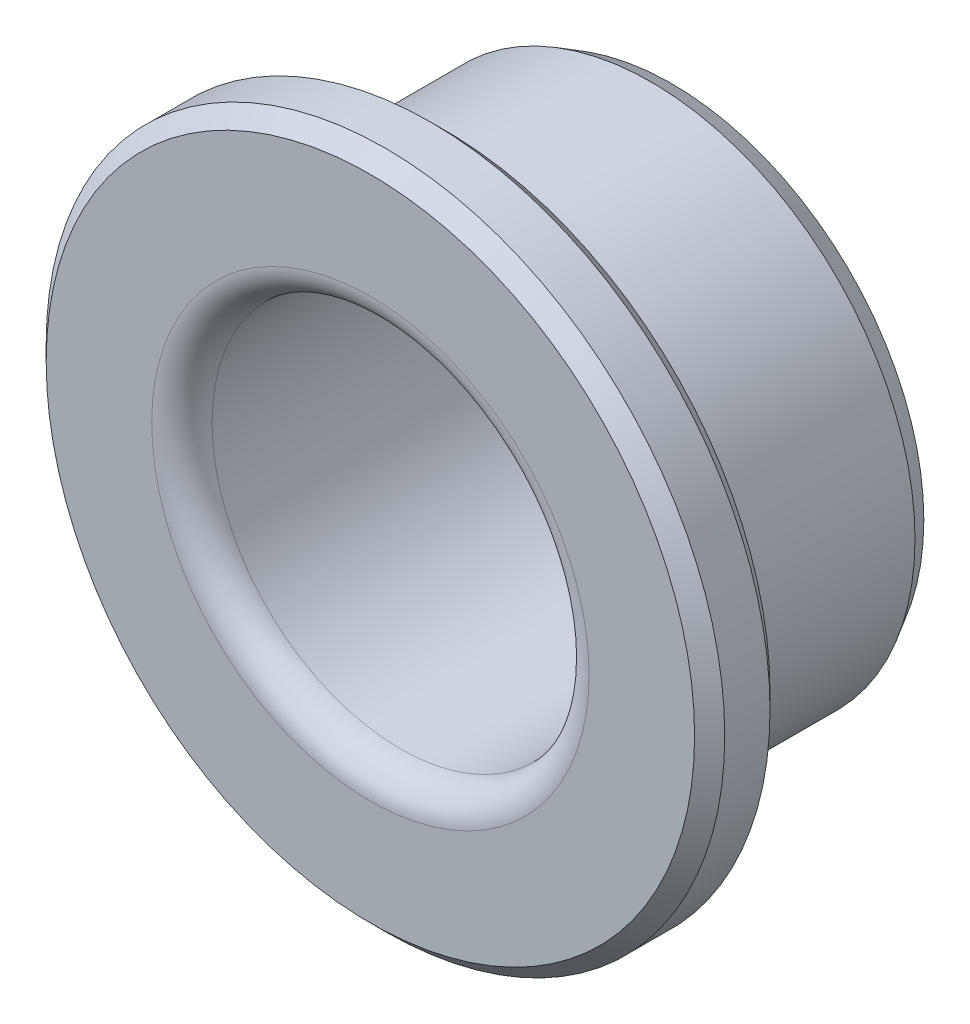
SolidWorks part; units mm, degrees
material "Plain Carbon Steel"
ref_plane "Front Plane" through (0, 0, 0) normal (0, 0, 1) x (1, 0, 0)
ref_plane "Top Plane" through (0, 0, 0) normal (0, 1, 0) x (1, 0, 0)
ref_plane "Right Plane" through (0, 0, 0) normal (1, 0, 0) x (0, 0, -1)
sketch "Body Profile Ø35" plane through (0, 0, 0) normal (0, 0, 1) x (1, 0, 0)
  circle A0 centre (0, 0) radius 17.5
  dimension "D1" = 35
extrude "Body Ø35" add sketch "Body Profile Ø35" along normal blind 15
sketch "Flange Profile Ø45" plane through (0, 0, 15) normal (0, 0, 1) x (1, 0, 0)
  circle A0 centre (0, 0) radius 22.5
  dimension "D1" = 45
extrude "Flange Ø45" add sketch "Flange Profile Ø45" along normal blind 5
chamfer "Body End Chamfer 0.8x60°" distance 0.8 angle 60 1 edges at (17.5, 0, 0)
sketch "Bore Profile Ø25" plane through (0, 0, 20) normal (0, 0, 1) x (1, 0, 0)
  circle A0 centre (0, 0) radius 12.5
  dimension "D1" = 25
extrude "Bore Ø25" cut sketch "Bore Profile Ø25" against normal through all
fillet "Flange Bore Fillet R2" radius 2 1 edges at (12.5, 0, 20)
chamfer "Flange Edge Chamfer 1x45°" distance 1 angle 45 2 edges at (22.5, 0, 15) (22.5, 0, 20)
fillet "Body Bore Fillet R1" radius 1 1 edges at (12.5, 0, 0)
